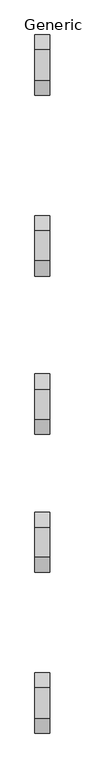
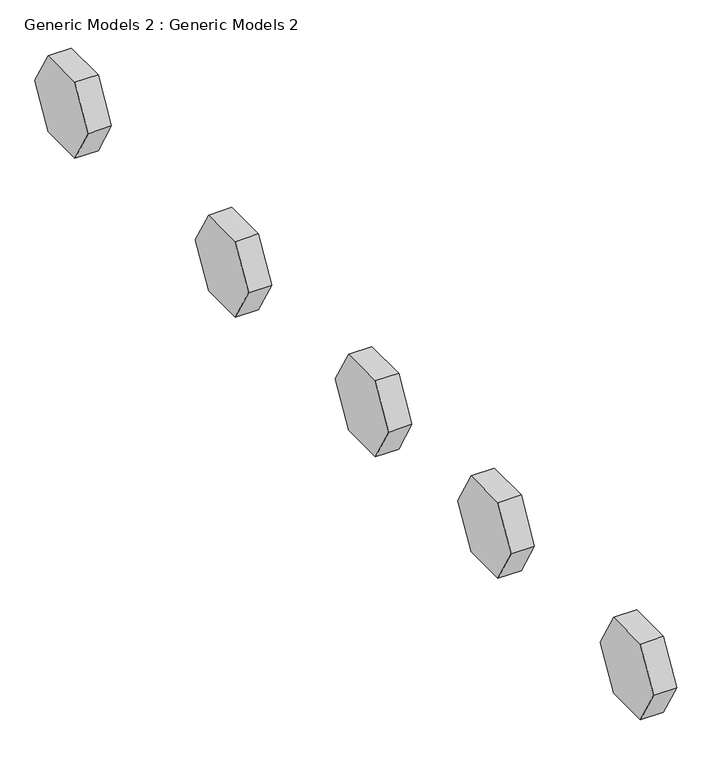
"""IFC4 building model written with IfcOpenShell, lengths in millimetres: proxy geometry, Generic Models 2 : Generic Models 2."""

from ifc_helpers import new_model, si_unit, frame, origin, place, context, project, spatial, polyline, outline, extrude, source, transform, mapped, element, save


def generic_models_2_generic_models_2_a0eb84b6(model_context):
    return source(origin(), model_context, "Body", "SweptSolid", [
        extrude(outline(polyline([(6462.3443296, 1289.9290861), (7071.9443296, 1289.9290861), (7376.7443296, 762.0), (7071.9443296, 234.0709139), (6462.3443296, 234.0709139), (6157.5443296, 762.0), (6462.3443296, 1289.9290861)])), frame((-6911.4872391, 0.0, 0.0), z_axis=(1.0, 0.0, 0.0), x_axis=(0.0, 1.0, 0.0)), (0.0, 0.0, 1.0), 304.8),
        extrude(outline(polyline([(2804.7443296, 1289.9290861), (3414.3443296, 1289.9290861), (3719.1443296, 762.0), (3414.3443296, 234.0709139), (2804.7443296, 234.0709139), (2499.9443296, 762.0), (2804.7443296, 1289.9290861)])), frame((-6911.4872391, 0.0, 0.0), z_axis=(1.0, 0.0, 0.0), x_axis=(0.0, 1.0, 0.0)), (0.0, 0.0, 1.0), 304.8),
        extrude(outline(polyline([(-395.6556704, 1289.9290861), (213.9443296, 1289.9290861), (518.7443296, 762.0), (213.9443296, 234.0709139), (-395.6556704, 234.0709139), (-700.4556704, 762.0), (-395.6556704, 1289.9290861)])), frame((-6911.4872391, 0.0, 0.0), z_axis=(1.0, 0.0, 0.0), x_axis=(0.0, 1.0, 0.0)), (0.0, 0.0, 1.0), 304.8),
        extrude(outline(polyline([(-3189.6556704, 1289.9290861), (-2580.0556704, 1289.9290861), (-2275.2556704, 762.0), (-2580.0556704, 234.0709139), (-3189.6556704, 234.0709139), (-3494.4556704, 762.0), (-3189.6556704, 1289.9290861)])), frame((-6911.4872391, 0.0, 0.0), z_axis=(1.0, 0.0, 0.0), x_axis=(0.0, 1.0, 0.0)), (0.0, 0.0, 1.0), 304.8),
        extrude(outline(polyline([(-6440.8556704, 1289.9290861), (-5831.2556704, 1289.9290861), (-5526.4556704, 762.0), (-5831.2556704, 234.0709139), (-6440.8556704, 234.0709139), (-6745.6556704, 762.0), (-6440.8556704, 1289.9290861)])), frame((-6911.4872391, 0.0, 0.0), z_axis=(1.0, 0.0, 0.0), x_axis=(0.0, 1.0, 0.0)), (0.0, 0.0, 1.0), 304.8),
    ])


if __name__ == "__main__":
    model = new_model("IFC4")
    model_context = context("Model", 3, world=origin())
    ifc_project = project(units=[si_unit("LENGTHUNIT", "METRE", prefix="MILLI")], contexts=[model_context])
    site = spatial("IfcSite", under=ifc_project)
    building = spatial("IfcBuilding", under=site)
    placement = place(None, origin())
    generic_models_2_generic_models_2_shape = generic_models_2_generic_models_2_a0eb84b6(model_context)
    element("IfcBuildingElementProxy", 1, Name="Generic Models 2 : Generic Models 2", ObjectType="Generic Models 2 : Generic Models 2", at=placement, inside=building, context=model_context, shape_type="MappedRepresentation", body=[
        mapped(generic_models_2_generic_models_2_shape, transform((0.0, 0.0, 0.0), x_axis=(1.0, 0.0, 0.0), y_axis=(0.0, 1.0, 0.0), z_axis=(0.0, 0.0, 1.0))),
    ])
    save(model, "model.ifc")

# Revit data of these elements
# Element 1 (IfcBuildingElementProxy, "Generic Models 2 : Generic Models 2")
#   Materials on its faces: "Clad - White", "Concrete Masonry Units"
# Materials
#   "Clad - White": class "Wood", colour RGB 242 242 238, transparency 0, Cost = 0
#   "Concrete Masonry Units": class "Masonry", colour RGB 227 227 227, transparency 0, Description = "Concrete masonry units", Cost = 0
